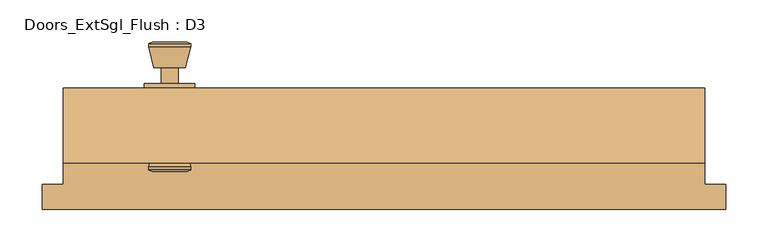
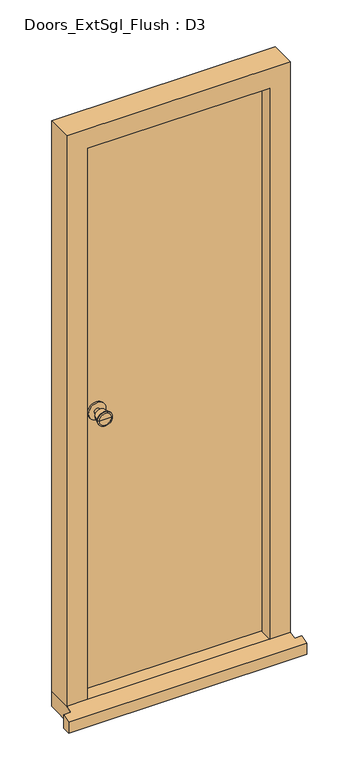
"""IFC4 building model written with IfcOpenShell, lengths in millimetres: door geometry, Doors_ExtSgl_Flush : D3."""

from ifc_helpers import new_model, si_unit, point, frame, frame_2d, origin, place, context, project, spatial, polyline, circle_curve, trimmed, segment, composite_curve, outline, extrude, faceted_brep, source, transform, mapped, element, save
from ifc_brep_helpers import plane_surface, cylinder_surface, revolved_surface, advanced_brep


def doors_extsgl_flush_d3_225e8ac6(model_context):
    return source(origin(), model_context, "Body", "SolidModel", [
        advanced_brep(
        [(-254.5, 95.3112, 1050.0), (-264.5, 95.3112, 1050.0), (-244.5, 95.3112, 1050.0), (-234.0241324, 144.3112, 1050.0), (-274.9758676, 144.3112, 1050.0), (-254.5, 144.3112, 1050.0), (-229.5, 142.4833319, 1050.0), (-279.5, 142.4833319, 1050.0), (-229.5, 139.0196537, 1050.0), (-279.5, 139.0196537, 1050.0), (-235.863764, 114.3112, 1050.0), (-273.136236, 114.3112, 1050.0), (-244.5, 114.3112, 1050.0), (-264.5, 114.3112, 1050.0)],
        [
            (0, 1),
            (1, 2, circle_curve(frame((-254.5, 95.3112, 1050.0), z_axis=(0.0, -1.0, 0.0), x_axis=(-1.0, 0.0, 0.0)), 10.0)),
            (2, 0),
            (2, 1, circle_curve(frame((-254.5, 95.3112, 1050.0), z_axis=(0.0, -1.0, 0.0), x_axis=(-1.0, 0.0, 0.0)), 10.0)),
            (3, 4, circle_curve(frame((-254.5, 144.3112, 1050.0), z_axis=(0.0, 1.0, 0.0), x_axis=(-1.0, 0.0, 0.0)), 20.4758676)),
            (4, 5),
            (5, 3),
            (4, 3, circle_curve(frame((-254.5, 144.3112, 1050.0), z_axis=(0.0, 1.0, 0.0), x_axis=(-1.0, 0.0, 0.0)), 20.4758676)),
            (6, 7, circle_curve(frame((-254.5, 142.4833319, 1050.0), z_axis=(0.0, 1.0, 0.0), x_axis=(-1.0, 0.0, 0.0)), 25.0)),
            (7, 4),
            (3, 6),
            (7, 6, circle_curve(frame((-254.5, 142.4833319, 1050.0), z_axis=(0.0, 1.0, 0.0), x_axis=(-1.0, 0.0, 0.0)), 25.0)),
            (8, 9, circle_curve(frame((-254.5, 139.0196537, 1050.0), z_axis=(0.0, 1.0, 0.0), x_axis=(-1.0, 0.0, 0.0)), 25.0)),
            (9, 7),
            (6, 8),
            (9, 8, circle_curve(frame((-254.5, 139.0196537, 1050.0), z_axis=(0.0, 1.0, 0.0), x_axis=(-1.0, 0.0, 0.0)), 25.0)),
            (10, 11, circle_curve(frame((-254.5, 114.3112, 1050.0), z_axis=(0.0, 1.0, 0.0), x_axis=(-1.0, 0.0, 0.0)), 18.636236)),
            (11, 9),
            (8, 10),
            (11, 10, circle_curve(frame((-254.5, 114.3112, 1050.0), z_axis=(0.0, 1.0, 0.0), x_axis=(-1.0, 0.0, 0.0)), 18.636236)),
            (12, 13, circle_curve(frame((-254.5, 114.3112, 1050.0), z_axis=(0.0, 1.0, 0.0), x_axis=(-1.0, 0.0, 0.0)), 10.0)),
            (13, 11),
            (10, 12),
            (13, 12, circle_curve(frame((-254.5, 114.3112, 1050.0), z_axis=(0.0, 1.0, 0.0), x_axis=(-1.0, 0.0, 0.0)), 10.0)),
            (1, 13),
            (12, 2),
        ],
        [
            plane_surface(frame((-254.5, 95.3112, 1050.0), z_axis=(0.0, -1.0, 0.0), x_axis=(-1.0, 0.0, 0.0))),
            plane_surface(frame((-254.5, 144.3112, 1050.0), z_axis=(0.0, 1.0, 0.0), x_axis=(-1.0, 0.0, 0.0))),
            revolved_surface(polyline([(-274.9758676, 144.3112, 1050.0), (-279.5, 142.4833319, 1050.0)]), (-254.5, 95.3112, 1050.0), (0.0, -1.0, 0.0)),
            cylinder_surface(frame((-254.5, 95.3112, 1050.0), z_axis=(0.0, -1.0, 0.0), x_axis=(-1.0, 0.0, 0.0)), 25.0),
            revolved_surface(polyline([(-279.5, 139.0196537, 1050.0), (-273.136236, 114.3112, 1050.0)]), (-254.5, 95.3112, 1050.0), (0.0, -1.0, 0.0)),
            plane_surface(frame((-254.5, 114.3112, 1050.0), z_axis=(0.0, -1.0, 0.0), x_axis=(-1.0, 0.0, 0.0))),
            cylinder_surface(frame((-254.5, 95.3112, 1050.0), z_axis=(0.0, -1.0, 0.0), x_axis=(-1.0, 0.0, 0.0)), 10.0),
        ],
        [
            (0, [[1, 2, 3]]),
            (0, [[-3, 4, -1]]),
            (1, [[5, 6, 7]]),
            (1, [[8, -7, -6]]),
            (2, [[9, 10, -5, 11]]),
            (2, [[12, -11, -8, -10]]),
            (3, [[13, 14, -9, 15]]),
            (3, [[16, -15, -12, -14]]),
            (4, [[17, 18, -13, 19]]),
            (4, [[20, -19, -16, -18]]),
            (5, [[21, 22, -17, 23]]),
            (5, [[24, -23, -20, -22]]),
            (6, [[-2, 25, -21, 26]]),
            (6, [[-4, -26, -24, -25]]),
        ],
    ),
        extrude(outline(composite_curve([segment(trimmed(circle_curve(frame_2d((1050.0, -254.5)), 30.0), [point((1050.0, -284.5))], [point((1050.0, -224.5))], False, "CARTESIAN"), True, "CONTINUOUS"), segment(trimmed(circle_curve(frame_2d((1050.0, -254.5)), 30.0), [point((1050.0, -224.5))], [point((1050.0, -284.5))], False, "CARTESIAN"), True, "CONTINUOUS")], self_intersect=False)), frame((0.0, 89.3112, 0.0), z_axis=(0.0, 1.0, 0.0), x_axis=(0.0, 0.0, 1.0)), (0.0, 0.0, 1.0), 6.0),
        advanced_brep(
        [(-254.5, 39.3112, 1050.0), (-244.5, 39.3112, 1050.0), (-264.5, 39.3112, 1050.0), (-234.0241324, -9.6888, 1050.0), (-254.5, -9.6888, 1050.0), (-274.9758676, -9.6888, 1050.0), (-229.5, -7.8609319, 1050.0), (-279.5, -7.8609319, 1050.0), (-229.5, -4.3972537, 1050.0), (-279.5, -4.3972537, 1050.0), (-235.863764, 20.3112, 1050.0), (-273.136236, 20.3112, 1050.0), (-244.5, 20.3112, 1050.0), (-264.5, 20.3112, 1050.0)],
        [
            (0, 1),
            (1, 2, circle_curve(frame((-254.5, 39.3112, 1050.0), z_axis=(0.0, 1.0, 0.0), x_axis=(-1.0, 0.0, 0.0)), 10.0)),
            (2, 0),
            (2, 1, circle_curve(frame((-254.5, 39.3112, 1050.0), z_axis=(0.0, 1.0, 0.0), x_axis=(-1.0, 0.0, 0.0)), 10.0)),
            (3, 4),
            (4, 5),
            (5, 3, circle_curve(frame((-254.5, -9.6888, 1050.0), z_axis=(0.0, -1.0, 0.0), x_axis=(-1.0, 0.0, 0.0)), 20.4758676)),
            (3, 5, circle_curve(frame((-254.5, -9.6888, 1050.0), z_axis=(0.0, -1.0, 0.0), x_axis=(-1.0, 0.0, 0.0)), 20.4758676)),
            (6, 3),
            (5, 7),
            (7, 6, circle_curve(frame((-254.5, -7.8609319, 1050.0), z_axis=(0.0, -1.0, 0.0), x_axis=(-1.0, 0.0, 0.0)), 25.0)),
            (6, 7, circle_curve(frame((-254.5, -7.8609319, 1050.0), z_axis=(0.0, -1.0, 0.0), x_axis=(-1.0, 0.0, 0.0)), 25.0)),
            (8, 6),
            (7, 9),
            (9, 8, circle_curve(frame((-254.5, -4.3972537, 1050.0), z_axis=(0.0, -1.0, 0.0), x_axis=(-1.0, 0.0, 0.0)), 25.0)),
            (8, 9, circle_curve(frame((-254.5, -4.3972537, 1050.0), z_axis=(0.0, -1.0, 0.0), x_axis=(-1.0, 0.0, 0.0)), 25.0)),
            (10, 8),
            (9, 11),
            (11, 10, circle_curve(frame((-254.5, 20.3112, 1050.0), z_axis=(0.0, -1.0, 0.0), x_axis=(-1.0, 0.0, 0.0)), 18.636236)),
            (10, 11, circle_curve(frame((-254.5, 20.3112, 1050.0), z_axis=(0.0, -1.0, 0.0), x_axis=(-1.0, 0.0, 0.0)), 18.636236)),
            (12, 10),
            (11, 13),
            (13, 12, circle_curve(frame((-254.5, 20.3112, 1050.0), z_axis=(0.0, -1.0, 0.0), x_axis=(-1.0, 0.0, 0.0)), 10.0)),
            (12, 13, circle_curve(frame((-254.5, 20.3112, 1050.0), z_axis=(0.0, -1.0, 0.0), x_axis=(-1.0, 0.0, 0.0)), 10.0)),
            (1, 12),
            (13, 2),
        ],
        [
            plane_surface(frame((-254.5, 39.3112, 1050.0), z_axis=(0.0, 1.0, 0.0), x_axis=(-1.0, 0.0, 0.0))),
            plane_surface(frame((-254.5, -9.6888, 1050.0), z_axis=(0.0, -1.0, 0.0), x_axis=(-1.0, 0.0, 0.0))),
            revolved_surface(polyline([(-274.9758676, -9.6888, 1050.0), (-279.5, -7.8609319, 1050.0)]), (-254.5, 39.3112, 1050.0), (0.0, 1.0, 0.0)),
            cylinder_surface(frame((-254.5, 39.3112, 1050.0), z_axis=(0.0, 1.0, 0.0), x_axis=(-1.0, 0.0, 0.0)), 25.0),
            revolved_surface(polyline([(-279.5, -4.3972537, 1050.0), (-273.136236, 20.3112, 1050.0)]), (-254.5, 39.3112, 1050.0), (0.0, 1.0, 0.0)),
            plane_surface(frame((-254.5, 20.3112, 1050.0), z_axis=(0.0, 1.0, 0.0), x_axis=(-1.0, 0.0, 0.0))),
            cylinder_surface(frame((-254.5, 39.3112, 1050.0), z_axis=(0.0, 1.0, 0.0), x_axis=(-1.0, 0.0, 0.0)), 10.0),
        ],
        [
            (0, [[1, 2, 3]]),
            (0, [[-3, 4, -1]]),
            (1, [[5, 6, 7]]),
            (1, [[-6, -5, 8]]),
            (2, [[9, -7, 10, 11]]),
            (2, [[-10, -8, -9, 12]]),
            (3, [[13, -11, 14, 15]]),
            (3, [[-14, -12, -13, 16]]),
            (4, [[17, -15, 18, 19]]),
            (4, [[-18, -16, -17, 20]]),
            (5, [[21, -19, 22, 23]]),
            (5, [[-22, -20, -21, 24]]),
            (6, [[25, -23, 26, -2]]),
            (6, [[-26, -24, -25, -4]]),
        ],
    ),
        extrude(outline(composite_curve([segment(trimmed(circle_curve(frame_2d((1050.0, -254.5)), 30.0), [point((1050.0, -284.5))], [point((1050.0, -224.5))], False, "CARTESIAN"), True, "CONTINUOUS"), segment(trimmed(circle_curve(frame_2d((1050.0, -254.5)), 30.0), [point((1050.0, -224.5))], [point((1050.0, -284.5))], False, "CARTESIAN"), True, "CONTINUOUS")], self_intersect=False)), frame((0.0, 39.3112, 0.0), z_axis=(0.0, 1.0, 0.0), x_axis=(0.0, 0.0, 1.0)), (0.0, 0.0, 1.0), 6.0),
        faceted_brep([(310.5, 0.3112, 54.5), (310.5, 42.3112, 54.5), (332.5, 42.3112, 54.5), (332.5, 89.3112, 54.5), (381.0, 89.3112, 54.5), (381.0, 0.3112, 54.5), (381.0, 0.3112, 2110.0), (-381.0, 0.3112, 2110.0), (-381.0, 0.3112, 54.5), (-310.5, 0.3112, 54.5), (-310.5, 0.3112, 2039.5), (310.5, 0.3112, 2039.5), (381.0, 89.3112, 2110.0), (332.5, 89.3112, 2061.5), (-332.5, 89.3112, 2061.5), (-332.5, 89.3112, 54.5), (-381.0, 89.3112, 54.5), (-381.0, 89.3112, 2110.0), (332.5, 42.3112, 2061.5), (310.5, 42.3112, 2039.5), (-310.5, 42.3112, 2039.5), (-310.5, 42.3112, 54.5), (-332.5, 42.3112, 54.5), (-332.5, 42.3112, 2061.5)], [[[0, 1, 2, 3, 4, 5]], [[5, 6, 7, 8, 9, 10, 11, 0]], [[4, 12, 6, 5]], [[3, 13, 14, 15, 16, 17, 12, 4]], [[2, 18, 13, 3]], [[1, 19, 20, 21, 22, 23, 18, 2]], [[0, 11, 19, 1]], [[10, 9, 21, 20]], [[9, 8, 16, 15, 22, 21]], [[17, 16, 8, 7]], [[23, 22, 15, 14]], [[12, 17, 7, 6]], [[18, 23, 14, 13]], [[11, 10, 20, 19]]]),
        extrude(outline(polyline([(329.5, 89.3112), (329.5, 45.3112), (-330.4250294, 45.3112), (-330.4250294, 89.3112), (329.5, 89.3112)])), frame((0.0, 0.0, 58.5), z_axis=(0.0, 0.0, 1.0), x_axis=(1.0, 0.0, 0.0)), (0.0, 0.0, 1.0), 2000.0),
        faceted_brep([(406.0, -54.6888, 0.0), (406.0, -24.6888, 0.0), (406.0, -24.6888, 47.2703282), (406.0, -54.6888, 38.5947221), (-406.0, -54.6888, 38.5947221), (-406.0, -24.6888, 47.2703282), (-406.0, -24.6888, 0.0), (-406.0, -54.6888, 0.0), (-381.0, -24.6888, 0.0), (-381.0, 89.3112, 0.0), (381.0, 89.3112, 0.0), (381.0, -24.6888, 0.0), (381.0, -24.6888, 47.2703282), (381.0, 0.3112, 54.5), (-381.0, 0.3112, 54.5), (-381.0, -24.6888, 47.2703282), (381.0, 89.3112, 54.5), (-381.0, 89.3112, 54.5)], [[[0, 1, 2, 3]], [[4, 5, 6, 7]], [[7, 6, 8, 9, 10, 11, 1, 0]], [[3, 4, 7, 0]], [[3, 2, 12, 13, 14, 15, 5, 4]], [[14, 13, 16, 17]], [[17, 16, 10, 9]], [[15, 14, 17, 9, 8]], [[8, 6, 5, 15]], [[11, 10, 16, 13, 12]], [[12, 2, 1, 11]]]),
    ])


if __name__ == "__main__":
    model = new_model("IFC4")
    model_context = context("Model", 3, world=origin())
    ifc_project = project(units=[si_unit("LENGTHUNIT", "METRE", prefix="MILLI")], contexts=[model_context])
    site = spatial("IfcSite", under=ifc_project)
    building = spatial("IfcBuilding", under=site)
    placement = place(None, origin())
    doors_extsgl_flush_d3_shape = doors_extsgl_flush_d3_225e8ac6(model_context)
    element("IfcDoor", 1, ObjectType="Doors_ExtSgl_Flush : D3", at=placement, inside=building, context=model_context, shape_type="MappedRepresentation", body=[
        mapped(doors_extsgl_flush_d3_shape, transform((0.0, 0.0, 0.0), x_axis=(1.0, 0.0, 0.0), y_axis=(0.0, 1.0, 0.0), z_axis=(0.0, 0.0, 1.0))),
    ])
    save(model, "model.ifc")

# Revit data of these elements
# Type "Doors_ExtSgl_Flush : D3"
#   Type Mark = "51"
#   Type Comments = "External Single"
#   Operation = "SingleSwingRight"
#   Construction Type Id = "MDOOR"
#   Keynote = "L20"
#   Analytic Construction = "Metal"
#   Wrap Layers (Int) from Ext = 177.5 mm
#   Wrap Layers (Ext) from Ext = 102.5 mm
#   Thickness = 44 mm
#   Rough Width = 762 mm
#   Rough Height = 2110 mm
#   O/A Frame Width = 64 mm
#   Heat Transfer Coefficient (U) = 3.7021 W/(m²·K)
#   Handle Z Distance = 1050 mm
#   FrameWidth = 42 mm
#   FrameOffset - External = 25 mm
#   FrameDepth = 89 mm
#   Door Panel Width = 659 mm
#   Door Panel Thickness = 44 mm
#   Door Panel Height = 2000 mm
#   Cill Thickness = 54.5 mm
#   Cill Projection = 30 mm
#   Handle X Distance = 75 mm
#   Height = 2110 mm
#   Structural Tolerance = 6.5 mm
#   Tolerance = 3 mm
#   Undercut = 4 mm
#   Width = 762 mm
#   Cill Extension = 25 mm
#   Cavity Closer Width = 50 mm
#   Cavity Closer Offset from Ext = 102.5 mm
#   Cavity Closer Depth = 85 mm
#   Vis - Ironmongery = yes
#   Vis - Cavity Closers = yes
#   Define Thermal Properties by = 1
#   Function = 1
#   Material Door = Door - Panel
#   Material Frame = Door - Frame/Mullion
#   Material Ironmongery = Door - Handle
#   Visual Light Transmittance = 0
#   Solar Heat Gain Coefficient = 0
#   Wall Closure = (empty or 0)
# Element 1 (IfcDoor, "Doors_ExtSgl_Flush : D3")
#   Materials on its faces: "Door - Handle", "Door - Frame/Mullion", "Door - Panel"
# Materials
#   "Door - Panel": class "Wood", colour RGB 210 159 95, transparency 0, Keynote = "L20", Cost = 0
#   "Door - Frame/Mullion": class "Wood", colour RGB 212 179 113, transparency 0, Keynote = "L20", Cost = 0
#   "Door - Handle": colour RGB 0 0 0, transparency 0, Keynote = "P21", Cost = 0
